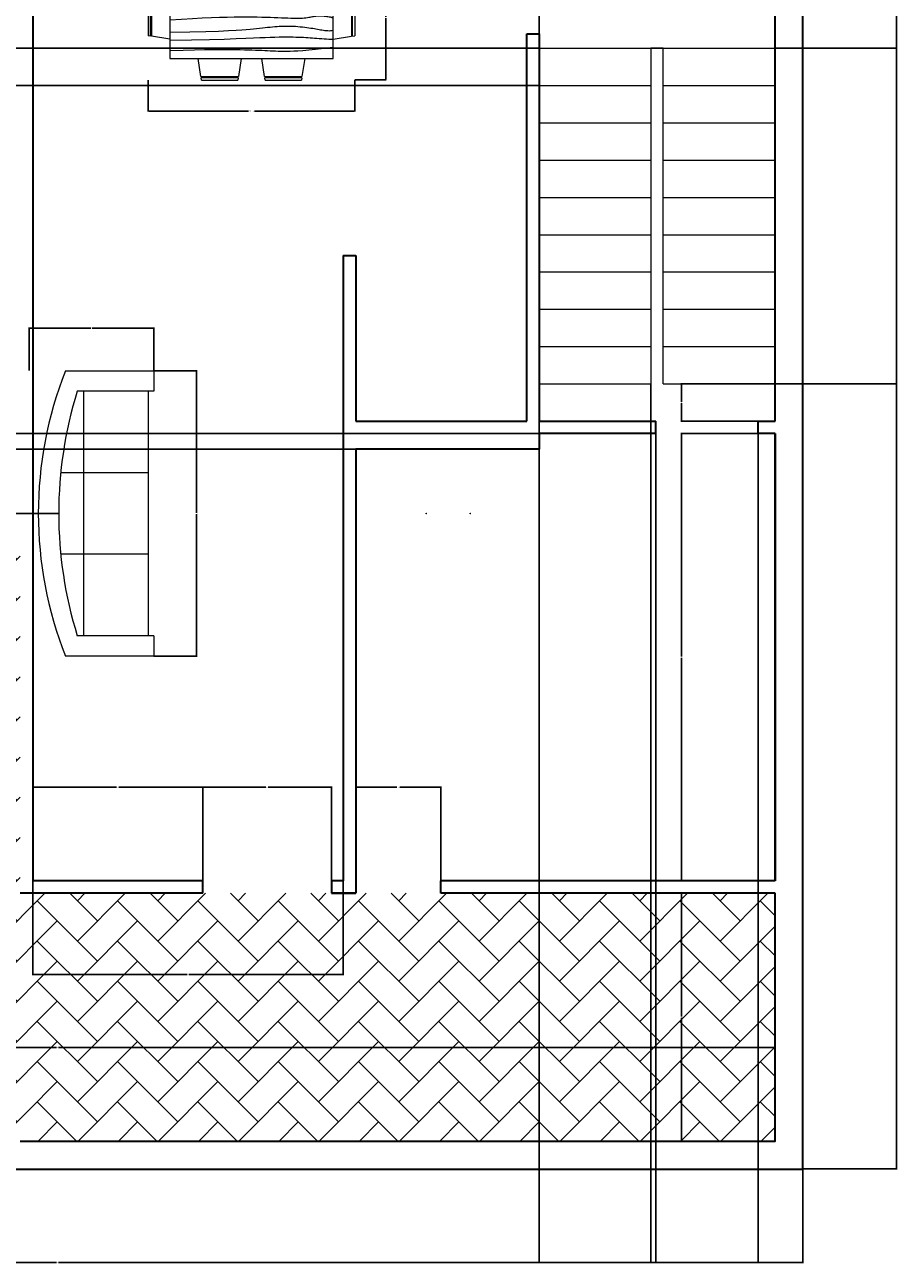
# Model space of a CAD drawing. Units: feet. Extents: x 2335 to 2876, y 491 to 1152.
# Tile 2 of 4: x 2595 to 2876, y 491 to 890. Entities that reach past the tile are written whole.
import ezdxf

# ---------------------------------------------------------------- set-up
doc = ezdxf.new("R2010")
doc.units = ezdxf.units.FT
for name, color, linetype, lineweight in [('A-ANNO-DIMS', 2, 'Continuous', 18), ('A-FLOR-STRS', 4, 'Continuous', 18), ('A-FURN', 8, 'Continuous', 18), ('A-WALL', 7, 'Continuous', 35), ('C-PROP', 3, 'Continuous', 35), ('C-PVMT-PATT', 252, 'Continuous', 13)]:
    doc.layers.add(name, color=color, linetype=linetype, lineweight=lineweight)
doc.styles.get("Standard").update_dxf_attribs({"font": 'arial.ttf'})
doc.dimstyles.get("Standard").update_dxf_attribs({"dimtxt": 0.18, "dimasz": 0.18, "dimexe": 0.18, "dimexo": 0.0625, "dimgap": 0.09, "dimtad": 0, "dimtih": 1, "dimtoh": 1, "dimdec": 4, "dimzin": 0, "dimdsep": 46, "dimlunit": 4, "dimtxsty": 'Standard', "dimcen": 0.09, "dimadec": 0, "dimazin": 0, "dimtfac": 1, "dimtdec": 4, "dimtofl": 0, "dimtmove": 0, "dimatfit": 3, "dimfxl": 1, "dimtolj": 1, "dimtzin": 0, "dimarcsym": 0})

# ---------------------------------------------------------------- blocks, each defined once
blk = doc.blocks.new('Dining Set - 36 x 72 in.')
for p, q in [((-22, 27.5), (-22.1562, 26.50042)), ((-22, 27.5), (-6, 27.5)), ((-5.8437, 26.49966), (-6, 27.5)), ((6, 27.5), (5.8438, 26.50042)), ((6, 27.5), (22, 27.5)), ((22.1563, 26.49966), (22, 27.5)), ((-22.2343, 26.00059), (-23.4847, 17.99762)), ((-22.2304, 26), (-5.7608, 26)), ((-5.8416, 26.5), (-22.1534, 26.5)), ((-4.5152, 17.99762), (-5.7655, 25.99926)), ((5.7657, 26.00059), (4.5153, 17.99762)), ((5.7696, 26), (22.2392, 26)), ((22.1584, 26.5), (5.8466, 26.5)), ((23.4848, 17.99762), (22.2345, 25.99926)), ((36, 18), (-36, 18)), ((-36, 18), (-36, -18)), ((36, -18), (36, 18)), ((-45.5, 8), (-44.5004, 8.15617)), ((-45.5, 8), (-45.5, -8)), ((-44.5, -8.15843), (-44.5, 8.15338)), ((-44.0006, 8.23428), (-35.9976, 9.48474)), ((-44, 8.23041), (-44, -8.23915)), ((44.0006, 8.23428), (35.9976, 9.48474)), ((44, 8.23041), (44, -8.23915)), ((44.5, -8.15843), (44.5, 8.15338)), ((45.5, 8), (44.5005, 8.15617)), ((45.5, 8), (45.5, -8)), ((-44.4997, -8.15631), (-45.5, -8)), ((-35.9976, -9.48476), (-43.9993, -8.2345)), ((35.9976, -9.48476), (43.9993, -8.2345)), ((44.4997, -8.15631), (45.5, -8)), ((-36, -18), (36, -18)), ((-22.2343, -26.0006), (-23.4847, -17.99762)), ((-4.5152, -17.99762), (-5.7655, -25.99928)), ((5.7657, -26.0006), (4.5153, -17.99762)), ((23.4848, -17.99762), (22.2345, -25.99928)), ((-22.2304, -26), (-5.7608, -26)), ((-22, -27.5), (-22.1562, -26.50044)), ((-5.8416, -26.5), (-22.1534, -26.5)), ((-5.8437, -26.49967), (-6, -27.5)), ((5.7696, -26), (22.2392, -26)), ((6, -27.5), (5.8438, -26.50044)), ((22.1584, -26.5), (5.8466, -26.5)), ((22.1563, -26.49967), (22, -27.5)), ((-22, -27.5), (-6, -27.5)), ((6, -27.5), (22, -27.5))]:
    blk.add_line(p, q)
for points in [[(-36, 15), (-31.1772, 14.97754), (-26.8079, 14.91406), (-22.8538, 14.81543), (-19.276, 14.6875), (-16.0362, 14.53613), (-13.0957, 14.36718), (-10.4159, 14.18652), (-7.9583, 14), (-5.6904, 13.81315), (-3.6035, 13.63021), (-1.6954, 13.45508), (0.0365, 13.29166), (1.5945, 13.14388), (2.9811, 13.01562), (4.1988, 12.9108), (5.25, 12.83333), (6.1393, 12.78613), (6.8802, 12.76823), (7.4883, 12.77767), (7.9792, 12.8125), (8.3685, 12.87077), (8.6719, 12.95052), (8.9049, 13.0498), (9.0833, 13.16666), (9.2205, 13.29899), (9.3216, 13.44401), (9.3895, 13.59879), (9.4271, 13.76041), (9.4373, 13.92594), (9.4232, 14.09245), (9.3875, 14.257), (9.3333, 14.41666), (9.2638, 14.56917), (9.1836, 14.71484), (9.0975, 14.85465), (9.0104, 14.98958), (8.9272, 15.1206), (8.8529, 15.2487), (8.7922, 15.37483), (8.75, 15.5), (8.7305, 15.62467), (8.7344, 15.74739), (8.7617, 15.86621), (8.8125, 15.97916), (8.8867, 16.08431), (8.9844, 16.17968), (9.1055, 16.26334), (9.25, 16.33333), (9.4189, 16.38802), (9.6172, 16.42708), (9.8506, 16.45052), (10.125, 16.45833), (10.4463, 16.45052), (10.8203, 16.42708), (11.2529, 16.38802), (11.75, 16.33333), (12.3184, 16.26318), (12.9694, 16.17838), (13.7151, 16.07991), (14.5677, 15.96875), (15.5395, 15.84586), (16.6426, 15.71224), (17.8893, 15.56884), (19.2917, 15.41666), (20.859, 15.25667), (22.5879, 15.08984), (24.4721, 14.91715), (26.5052, 14.73958), (28.6809, 14.5581), (30.9929, 14.3737), (33.4347, 14.18733), (36, 14)], [(-36, 10), (-28.9766, 10.14274), (-23.1725, 10.20442), (-18.4241, 10.19775), (-14.5677, 10.13541), (-11.4399, 10.03011), (-8.877, 9.89453), (-6.7154, 9.74137), (-4.7917, 9.58333), (-2.9698, 9.43082), (-1.2246, 9.28515), (0.4415, 9.14534), (2.026, 9.01041), (3.5266, 8.87939), (4.9408, 8.7513), (6.266, 8.62516), (7.5, 8.5), (8.6411, 8.37549), (9.6914, 8.2539), (10.6538, 8.13818), (11.5312, 8.03125), (12.3267, 7.93603), (13.043, 7.85547), (13.6831, 7.79248), (14.25, 7.75), (14.7471, 7.7303), (15.1797, 7.73307), (15.5537, 7.75732), (15.875, 7.80208), (16.1494, 7.86637), (16.3828, 7.94922), (16.5811, 8.04964), (16.75, 8.16666), (16.8944, 8.29915), (17.0143, 8.44531), (17.1089, 8.60319), (17.1771, 8.77083), (17.218, 8.94629), (17.2305, 9.1276), (17.2137, 9.31282), (17.1667, 9.5), (17.0895, 9.6875), (16.987, 9.875), (16.8649, 10.0625), (16.7292, 10.25), (16.5856, 10.4375), (16.4401, 10.625), (16.2985, 10.8125), (16.1667, 11), (16.05, 11.18733), (15.9518, 11.3737), (15.8752, 11.5581), (15.8229, 11.73958), (15.798, 11.91715), (15.8034, 12.08984), (15.842, 12.25667), (15.9167, 12.41666), (16.0295, 12.56836), (16.1784, 12.70833), (16.3605, 12.83268), (16.5729, 12.9375), (16.8127, 13.01888), (17.0768, 13.07291), (17.3625, 13.0957), (17.6667, 13.08333), (17.9894, 13.03312), (18.3418, 12.94726), (18.7382, 12.82918), (19.1927, 12.68229), (19.7195, 12.51001), (20.3327, 12.31575), (21.0465, 12.10294), (21.875, 11.875), (22.8357, 11.63354), (23.959, 11.37304), (25.2786, 11.08618), (26.8282, 10.76562), (28.6414, 10.40405), (30.752, 9.99414), (33.1936, 9.52856), (36, 9)], [(-36, 5.5), (-30.7157, 5.3348), (-26.069, 5.20963), (-21.9946, 5.11767), (-18.4271, 5.05208), (-15.3009, 5.00602), (-12.5508, 4.97265), (-10.1112, 4.94515), (-7.9167, 4.91666), (-5.909, 4.88167), (-4.0586, 4.83984), (-2.3429, 4.79215), (-0.7396, 4.73958), (0.7739, 4.6831), (2.22, 4.6237), (3.6213, 4.56233), (5, 4.5), (6.373, 4.43782), (7.7344, 4.3776), (9.0723, 4.32129), (10.375, 4.27083), (11.6309, 4.22819), (12.8281, 4.19531), (13.9551, 4.17415), (15, 4.16666), (15.954, 4.17448), (16.819, 4.19791), (17.6001, 4.23698), (18.3021, 4.29166), (18.9299, 4.36198), (19.4883, 4.44791), (19.9823, 4.54948), (20.4167, 4.66666), (20.7969, 4.79899), (21.1302, 4.94401), (21.4245, 5.09879), (21.6875, 5.26041), (21.9271, 5.42594), (22.1511, 5.59245), (22.3672, 5.757), (22.5834, 5.91666), (22.8065, 6.06868), (23.0404, 6.21093), (23.2879, 6.34147), (23.5521, 6.45833), (23.8358, 6.55957), (24.142, 6.64323), (24.4735, 6.70735), (24.8334, 6.75), (25.2235, 6.76969), (25.642, 6.76692), (26.0858, 6.74267), (26.5521, 6.69791), (27.0379, 6.63362), (27.5404, 6.55078), (28.0565, 6.45036), (28.5834, 6.33333), (29.1242, 6.19987), (29.7071, 6.04687), (30.3661, 5.87044), (31.1354, 5.66666), (32.0493, 5.43164), (33.142, 5.16146), (34.4475, 4.85221), (36, 4.5)], [(-36, -1), (-30.7915, -0.6591), (-26.0195, -0.38216), (-21.6519, -0.16284), (-17.6563, 0.00521), (-14.0005, 0.12833), (-10.6523, 0.21289), (-7.5796, 0.26522), (-4.75, 0.29166), (-2.134, 0.29793), (0.2878, 0.28711), (2.5317, 0.26163), (4.6146, 0.22396), (6.5529, 0.17651), (8.3633, 0.12174), (10.0623, 0.06209), (11.6667, 0), (13.1899, -0.06201), (14.6341, -0.1211), (15.9982, -0.17432), (17.2813, -0.21875), (18.4823, -0.25147), (19.6003, -0.26953), (20.6343, -0.27002), (21.5834, -0.25), (22.4481, -0.20768), (23.2357, -0.14584), (23.9549, -0.06836), (24.6146, 0.02083), (25.2235, 0.11784), (25.7904, 0.21875), (26.3241, 0.31966), (26.8334, 0.41666), (27.3265, 0.50618), (27.8099, 0.58593), (28.2894, 0.65397), (28.7709, 0.70833), (29.2601, 0.74707), (29.763, 0.76823), (30.2855, 0.76985), (30.8334, 0.75), (31.4088, 0.70784), (31.9994, 0.64713), (32.589, 0.57275), (33.1615, 0.48958), (33.7008, 0.4025), (34.1908, 0.3164), (34.6153, 0.23616), (34.9584, 0.16666), (35.2099, 0.11165), (35.3848, 0.07031), (35.504, 0.04069), (35.5886, 0.02083), (35.6594, 0.00879), (35.7377, 0.0026), (35.8442, 0.00032), (36, 0)], [(-36, -6.5), (-27.1843, -6.31267), (-20.084, -6.1263), (-14.469, -5.9419), (-10.1094, -5.76042), (-6.7752, -5.58285), (-4.2363, -5.41016), (-2.2629, -5.24333), (-0.625, -5.08334), (0.8708, -4.93099), (2.2715, -4.78646), (3.5872, -4.64974), (4.8281, -4.52084), (6.0046, -4.39974), (7.127, -4.28646), (8.2053, -4.18099), (9.25, -4.08334), (10.2705, -3.99382), (11.2734, -3.91407), (12.2647, -3.84603), (13.25, -3.79167), (14.2354, -3.75293), (15.2266, -3.73177), (16.2295, -3.73015), (17.25, -3.75), (18.2912, -3.79248), (19.3451, -3.85547), (20.4009, -3.93604), (21.4479, -4.03125), (22.4754, -4.13819), (23.4727, -4.25391), (24.4289, -4.37549), (25.3334, -4.5), (26.1785, -4.62492), (26.9694, -4.74935), (27.7145, -4.87281), (28.4219, -4.99479), (29.1, -5.11483), (29.7572, -5.23242), (30.4016, -5.34709), (31.0417, -5.45834), (31.6837, -5.56437), (32.3262, -5.65821), (32.9658, -5.73153), (33.599, -5.77604), (34.2224, -5.78345), (34.8327, -5.74545), (35.4264, -5.65373), (36, -5.5)], [(-36, -10), (-26.4022, -9.81299), (-18.4675, -9.62891), (-11.9839, -9.45069), (-6.7396, -9.28125), (-2.5226, -9.12354), (0.8789, -8.98047), (3.6769, -8.85498), (6.0833, -8.75), (8.2767, -8.66765), (10.3021, -8.60677), (12.1712, -8.56543), (13.8958, -8.54167), (15.4876, -8.53353), (16.9583, -8.53907), (18.3197, -8.55632), (19.5834, -8.58334), (20.7616, -8.61841), (21.8685, -8.66081), (22.9188, -8.71004), (23.9271, -8.76563), (24.9081, -8.82707), (25.8763, -8.89388), (26.8465, -8.96558), (27.8334, -9.04167), (28.8474, -9.12118), (29.8828, -9.20117), (30.93, -9.27824), (31.9792, -9.34896), (33.0205, -9.40991), (34.0443, -9.45768), (35.0407, -9.48885), (36, -9.5)], [(-36, -14.5), (-30.0881, -14.33513), (-25.0332, -14.21224), (-20.7312, -14.12647), (-17.0781, -14.07292), (-13.97, -14.04671), (-11.3027, -14.04297), (-8.9724, -14.05681), (-6.875, -14.08334), (-4.9224, -14.11833), (-3.0905, -14.16016), (-1.3709, -14.20785), (0.2448, -14.26042), (1.7647, -14.3169), (3.1973, -14.3763), (4.5507, -14.43767), (5.8333, -14.5), (7.0554, -14.5621), (8.235, -14.62175), (9.3922, -14.67652), (10.5469, -14.72396), (11.7192, -14.76164), (12.929, -14.78711), (14.1965, -14.79794), (15.5417, -14.79167), (16.9933, -14.76424), (18.6152, -14.70508), (20.4804, -14.60197), (22.6615, -14.44271), (25.2312, -14.21509), (28.2624, -13.9069), (31.8277, -13.50594), (36, -13)]]:
    blk.add_lwpolyline(points)
blk = doc.blocks.new('Sofa - Roundback 7 ft.')
for p, q in [((-12.00002, -32.4421), (-12.00003, -6.5971)), ((11.99997, -32.4421), (11.99998, -6.5971)), ((-36.000027, -34), (-36.000027, -11.4696)), ((-35.999844, -13.3819), (35.9998, -13.3819)), ((35.99998, -34), (35.99998, -11.4696)), ((-36.000027, -32.4421), (35.99998, -32.4421))]:
    blk.add_line(p, q)
for points in [[(-36.000027, -34), (-42.000027, -34), (-42.000027, -8)], [(41.99998, -8), (41.99998, -34), (35.99998, -34)]]:
    blk.add_lwpolyline(points)
for centre, radius, start, end in [((0, -114.25), 114.25, 68.43141, 111.5686), ((-0.00001, -127.1968), 121.1968, 72.72033, 107.2797)]:
    blk.add_arc(centre, radius, start, end)
blk = doc.blocks.new('*D20')
at = {"layer": 'A-ANNO-DIMS', "color": 0, "lineweight": -2, "transparency": 16777216}
for p, q in [((2634.96, 871.96), (2634.96, 861.86)), ((2701.49, 871.96), (2701.49, 861.86)), ((2635.14, 862.04), (2667.26, 862.04)), ((2701.31, 862.04), (2669.2, 862.04))]:
    blk.add_line(p, q, dxfattribs=at)
at = {"layer": 'A-ANNO-DIMS', "color": 0, "transparency": 16777216}
for points in [[(2635.14, 862.07), (2635.14, 862.01), (2634.96, 862.04)], [(2701.31, 862.07), (2701.31, 862.01), (2701.49, 862.04)]]:
    blk.add_solid(points, dxfattribs=at)
at = {"layer": 'Defpoints', "color": 0, "transparency": 16777216}
for p in [(2634.96, 872.02), (2701.49, 872.02), (2701.49, 862.04)]:
    blk.add_point(p, dxfattribs=at)
at = {"layer": 'A-ANNO-DIMS', "color": 0, "transparency": 16777216, "insert": (2668.23, 862.04), "char_height": 0.18, "attachment_point": 5}
blk.add_mtext('\\A1;DINING SET 67', dxfattribs=at)
blk = doc.blocks.new('*D21')
at = {"layer": 'A-ANNO-DIMS', "color": 0, "lineweight": -2, "transparency": 16777216}
for p, q in [((2701.56, 912.23), (2711.65, 912.23)), ((2711.47, 912.05), (2711.47, 892.31)), ((2711.47, 872.2), (2711.47, 891.94)), ((2701.56, 872.02), (2711.65, 872.02))]:
    blk.add_line(p, q, dxfattribs=at)
at = {"layer": 'A-ANNO-DIMS', "color": 0, "transparency": 16777216}
for points in [[(2711.44, 912.05), (2711.5, 912.05), (2711.47, 912.23)], [(2711.44, 872.2), (2711.5, 872.2), (2711.47, 872.02)]]:
    blk.add_solid(points, dxfattribs=at)
at = {"layer": 'Defpoints', "color": 0, "transparency": 16777216}
for p in [(2701.49, 912.23), (2711.47, 912.23), (2701.49, 872.02)]:
    blk.add_point(p, dxfattribs=at)
at = {"layer": 'A-ANNO-DIMS', "color": 0, "transparency": 16777216, "insert": (2711.47, 892.13), "char_height": 0.18, "attachment_point": 5}
blk.add_mtext('\\A1;40', dxfattribs=at)
blk = doc.blocks.new('*D22')
at = {"layer": 'A-ANNO-DIMS', "color": 0, "lineweight": -2, "transparency": 16777216}
for p, q in [((2636.85, 778.42), (2650.74, 778.42)), ((2650.56, 778.24), (2650.56, 732.68)), ((2650.56, 686.75), (2650.56, 732.31)), ((2636.85, 686.57), (2650.74, 686.57))]:
    blk.add_line(p, q, dxfattribs=at)
at = {"layer": 'A-ANNO-DIMS', "color": 0, "transparency": 16777216}
for points in [[(2650.53, 778.24), (2650.59, 778.24), (2650.56, 778.42)], [(2650.53, 686.75), (2650.59, 686.75), (2650.56, 686.57)]]:
    blk.add_solid(points, dxfattribs=at)
at = {"layer": 'Defpoints', "color": 0, "transparency": 16777216}
for p in [(2636.79, 778.42), (2650.56, 778.42), (2636.79, 686.57)]:
    blk.add_point(p, dxfattribs=at)
at = {"layer": 'A-ANNO-DIMS', "color": 0, "transparency": 16777216, "insert": (2650.56, 732.49), "char_height": 0.18, "attachment_point": 5}
blk.add_mtext('\\A1;SOFA 92', dxfattribs=at)
blk = doc.blocks.new('*D23')
at = {"layer": 'A-ANNO-DIMS', "color": 0, "lineweight": -2, "transparency": 16777216}
for p, q in [((2596.69, 778.48), (2596.69, 792.37)), ((2596.87, 792.19), (2616.52, 792.19)), ((2636.61, 792.19), (2616.96, 792.19)), ((2636.79, 778.48), (2636.79, 792.37))]:
    blk.add_line(p, q, dxfattribs=at)
at = {"layer": 'A-ANNO-DIMS', "color": 0, "transparency": 16777216}
for points in [[(2596.87, 792.22), (2596.87, 792.16), (2596.69, 792.19)], [(2636.61, 792.22), (2636.61, 792.16), (2636.79, 792.19)]]:
    blk.add_solid(points, dxfattribs=at)
at = {"layer": 'Defpoints', "color": 0, "transparency": 16777216}
for p in [(2596.69, 792.19), (2596.69, 778.42), (2636.79, 778.42)]:
    blk.add_point(p, dxfattribs=at)
at = {"layer": 'A-ANNO-DIMS', "color": 0, "transparency": 16777216, "insert": (2616.74, 792.19), "char_height": 0.18, "attachment_point": 5}
blk.add_mtext('\\A1;40', dxfattribs=at)
blk = doc.blocks.new('*D24')
at = {"layer": 'A-ANNO-DIMS', "color": 0, "lineweight": -2, "transparency": 16777216}
for p, q in [((2365.8, 521.42), (2365.8, 491.16)), ((2845.8, 521.42), (2845.8, 491.16)), ((2365.98, 491.34), (2605.5, 491.34)), ((2845.62, 491.34), (2606.09, 491.34))]:
    blk.add_line(p, q, dxfattribs=at)
at = {"layer": 'A-ANNO-DIMS', "color": 0, "transparency": 16777216}
for points in [[(2365.98, 491.37), (2365.98, 491.31), (2365.8, 491.34)], [(2845.62, 491.37), (2845.62, 491.31), (2845.8, 491.34)]]:
    blk.add_solid(points, dxfattribs=at)
at = {"layer": 'Defpoints', "color": 0, "transparency": 16777216}
for p in [(2365.8, 521.49), (2845.8, 521.49), (2845.8, 491.34)]:
    blk.add_point(p, dxfattribs=at)
at = {"layer": 'A-ANNO-DIMS', "color": 0, "transparency": 16777216, "insert": (2605.8, 491.34), "char_height": 0.18, "attachment_point": 5}
blk.add_mtext('\\A1;480', dxfattribs=at)
blk = doc.blocks.new('*D25')
at = {"layer": 'A-ANNO-DIMS', "color": 0, "lineweight": -2, "transparency": 16777216}
for p, q in [((2845.86, 1121.49), (2876.13, 1121.49)), ((2875.95, 1121.31), (2875.95, 821.67)), ((2875.95, 521.67), (2875.95, 821.31)), ((2845.86, 521.49), (2876.13, 521.49))]:
    blk.add_line(p, q, dxfattribs=at)
at = {"layer": 'A-ANNO-DIMS', "color": 0, "transparency": 16777216}
for points in [[(2875.92, 1121.31), (2875.98, 1121.31), (2875.95, 1121.49)], [(2875.92, 521.67), (2875.98, 521.67), (2875.95, 521.49)]]:
    blk.add_solid(points, dxfattribs=at)
at = {"layer": 'Defpoints', "color": 0, "transparency": 16777216}
for p in [(2845.8, 1121.49), (2875.95, 1121.49), (2845.8, 521.49)]:
    blk.add_point(p, dxfattribs=at)
at = {"layer": 'A-ANNO-DIMS', "color": 0, "transparency": 16777216, "insert": (2875.95, 821.49), "char_height": 0.18, "attachment_point": 5}
blk.add_mtext('\\A1;600', dxfattribs=at)
blk = doc.blocks.new('*D26')
at = {"layer": 'A-ANNO-DIMS', "color": 0, "lineweight": -2, "transparency": 16777216}
for p, q in [((2374.8, 530.55), (2374.8, 560.82)), ((2374.98, 560.64), (2605.51, 560.64)), ((2836.62, 560.64), (2606.09, 560.64)), ((2836.8, 530.55), (2836.8, 560.82))]:
    blk.add_line(p, q, dxfattribs=at)
at = {"layer": 'A-ANNO-DIMS', "color": 0, "transparency": 16777216}
for points in [[(2374.98, 560.67), (2374.98, 560.61), (2374.8, 560.64)], [(2836.62, 560.67), (2836.62, 560.61), (2836.8, 560.64)]]:
    blk.add_solid(points, dxfattribs=at)
at = {"layer": 'Defpoints', "color": 0, "transparency": 16777216}
for p in [(2836.8, 560.64), (2374.8, 530.49), (2836.8, 530.49)]:
    blk.add_point(p, dxfattribs=at)
at = {"layer": 'A-ANNO-DIMS', "color": 0, "transparency": 16777216, "insert": (2605.8, 560.64), "char_height": 0.18, "attachment_point": 5}
blk.add_mtext('\\A1;462', dxfattribs=at)
blk = doc.blocks.new('*D30')
at = {"layer": 'A-ANNO-DIMS', "color": 0, "lineweight": -2, "transparency": 16777216}
for p, q in [((2836.73, 610.23), (2806.47, 610.23)), ((2806.65, 610.05), (2806.65, 570.54)), ((2806.65, 530.67), (2806.65, 570.17)), ((2836.73, 530.49), (2806.47, 530.49))]:
    blk.add_line(p, q, dxfattribs=at)
at = {"layer": 'A-ANNO-DIMS', "color": 0, "transparency": 16777216}
for points in [[(2806.62, 610.05), (2806.68, 610.05), (2806.65, 610.23)], [(2806.62, 530.67), (2806.68, 530.67), (2806.65, 530.49)]]:
    blk.add_solid(points, dxfattribs=at)
at = {"layer": 'Defpoints', "color": 0, "transparency": 16777216}
for p in [(2806.65, 610.23), (2836.8, 610.23), (2836.8, 530.49)]:
    blk.add_point(p, dxfattribs=at)
at = {"layer": 'A-ANNO-DIMS', "color": 0, "transparency": 16777216, "insert": (2806.65, 570.36), "char_height": 0.18, "attachment_point": 5}
blk.add_mtext('\\A1;79.74', dxfattribs=at)
blk = doc.blocks.new('*D31')
at = {"layer": 'A-ANNO-DIMS', "color": 0, "lineweight": -2, "transparency": 16777216}
for p, q in [((2597.8, 614.16), (2597.8, 583.9)), ((2697.8, 614.16), (2697.8, 583.9)), ((2597.98, 584.08), (2647.52, 584.08)), ((2697.62, 584.08), (2648.08, 584.08))]:
    blk.add_line(p, q, dxfattribs=at)
at = {"layer": 'A-ANNO-DIMS', "color": 0, "transparency": 16777216}
for points in [[(2597.98, 584.11), (2597.98, 584.05), (2597.8, 584.08)], [(2697.62, 584.11), (2697.62, 584.05), (2697.8, 584.08)]]:
    blk.add_solid(points, dxfattribs=at)
at = {"layer": 'Defpoints', "color": 0, "transparency": 16777216}
for p in [(2597.8, 614.23), (2697.8, 614.23), (2597.8, 584.08)]:
    blk.add_point(p, dxfattribs=at)
at = {"layer": 'A-ANNO-DIMS', "color": 0, "transparency": 16777216, "insert": (2647.8, 584.08), "char_height": 0.18, "attachment_point": 5}
blk.add_mtext('\\A1;100', dxfattribs=at)
blk = doc.blocks.new('*D32')
at = {"layer": 'A-ANNO-DIMS', "color": 0, "lineweight": -2, "transparency": 16777216}
for p, q in [((2597.8, 614.29), (2597.8, 644.56)), ((2597.98, 644.38), (2624.79, 644.38)), ((2652.4, 644.38), (2625.58, 644.38)), ((2652.58, 614.29), (2652.58, 644.56))]:
    blk.add_line(p, q, dxfattribs=at)
at = {"layer": 'A-ANNO-DIMS', "color": 0, "transparency": 16777216}
for points in [[(2597.98, 644.41), (2597.98, 644.35), (2597.8, 644.38)], [(2652.4, 644.41), (2652.4, 644.35), (2652.58, 644.38)]]:
    blk.add_solid(points, dxfattribs=at)
at = {"layer": 'Defpoints', "color": 0, "transparency": 16777216}
for p in [(2652.58, 644.38), (2597.8, 614.23), (2652.58, 614.23)]:
    blk.add_point(p, dxfattribs=at)
at = {"layer": 'A-ANNO-DIMS', "color": 0, "transparency": 16777216, "insert": (2625.19, 644.38), "char_height": 0.18, "attachment_point": 5}
blk.add_mtext('\\A1;54.78', dxfattribs=at)
blk = doc.blocks.new('*D33')
at = {"layer": 'A-ANNO-DIMS', "color": 0, "lineweight": -2, "transparency": 16777216}
for p, q in [((2652.58, 614.29), (2652.58, 644.56)), ((2652.76, 644.38), (2672.9, 644.38)), ((2693.81, 644.38), (2673.66, 644.38)), ((2693.99, 614.29), (2693.99, 644.56))]:
    blk.add_line(p, q, dxfattribs=at)
at = {"layer": 'A-ANNO-DIMS', "color": 0, "transparency": 16777216}
for points in [[(2652.76, 644.41), (2652.76, 644.35), (2652.58, 644.38)], [(2693.81, 644.41), (2693.81, 644.35), (2693.99, 644.38)]]:
    blk.add_solid(points, dxfattribs=at)
at = {"layer": 'Defpoints', "color": 0, "transparency": 16777216}
for p in [(2693.99, 644.38), (2652.58, 614.23), (2693.99, 614.23)]:
    blk.add_point(p, dxfattribs=at)
at = {"layer": 'A-ANNO-DIMS', "color": 0, "transparency": 16777216, "insert": (2673.28, 644.38), "char_height": 0.18, "attachment_point": 5}
blk.add_mtext('\\A1;41.41', dxfattribs=at)
blk = doc.blocks.new('*D34')
at = {"layer": 'A-ANNO-DIMS', "color": 0, "lineweight": -2, "transparency": 16777216}
for p, q in [((2701.8, 614.29), (2701.8, 644.56)), ((2701.98, 644.38), (2715.03, 644.38)), ((2729, 644.38), (2715.96, 644.38)), ((2729.18, 614.29), (2729.18, 644.56))]:
    blk.add_line(p, q, dxfattribs=at)
at = {"layer": 'A-ANNO-DIMS', "color": 0, "transparency": 16777216}
for points in [[(2701.98, 644.41), (2701.98, 644.35), (2701.8, 644.38)], [(2729, 644.41), (2729, 644.35), (2729.18, 644.38)]]:
    blk.add_solid(points, dxfattribs=at)
at = {"layer": 'Defpoints', "color": 0, "transparency": 16777216}
for p in [(2729.18, 644.38), (2701.8, 614.23), (2729.18, 614.23)]:
    blk.add_point(p, dxfattribs=at)
at = {"layer": 'A-ANNO-DIMS', "color": 0, "transparency": 16777216, "insert": (2715.49, 644.38), "char_height": 0.18, "attachment_point": 5}
blk.add_mtext('\\A1;27.386', dxfattribs=at)
blk = doc.blocks.new('*D35')
at = {"layer": 'A-ANNO-DIMS', "color": 0, "lineweight": -2, "transparency": 16777216}
for p, q in [((2836.73, 758.23), (2806.47, 758.23)), ((2806.65, 758.05), (2806.65, 686.41)), ((2806.65, 614.41), (2806.65, 686.05)), ((2836.73, 614.23), (2806.47, 614.23))]:
    blk.add_line(p, q, dxfattribs=at)
at = {"layer": 'A-ANNO-DIMS', "color": 0, "transparency": 16777216}
for points in [[(2806.62, 758.05), (2806.68, 758.05), (2806.65, 758.23)], [(2806.62, 614.41), (2806.68, 614.41), (2806.65, 614.23)]]:
    blk.add_solid(points, dxfattribs=at)
at = {"layer": 'Defpoints', "color": 0, "transparency": 16777216}
for p in [(2806.65, 758.23), (2836.8, 758.23), (2836.8, 614.23)]:
    blk.add_point(p, dxfattribs=at)
at = {"layer": 'A-ANNO-DIMS', "color": 0, "transparency": 16777216, "insert": (2806.65, 686.23), "char_height": 0.18, "attachment_point": 5}
blk.add_mtext('\\A1;144', dxfattribs=at)
blk = doc.blocks.new('*D37')
at = {"layer": 'A-ANNO-DIMS', "color": 0, "lineweight": -2, "transparency": 16777216}
for p, q in [((2760.88, 882.29), (2760.88, 1151.82)), ((2761.06, 1151.64), (2798.45, 1151.64)), ((2836.62, 1151.64), (2799.23, 1151.64)), ((2836.8, 882.29), (2836.8, 1151.82))]:
    blk.add_line(p, q, dxfattribs=at)
at = {"layer": 'A-ANNO-DIMS', "color": 0, "transparency": 16777216}
for points in [[(2761.06, 1151.67), (2761.06, 1151.61), (2760.88, 1151.64)], [(2836.62, 1151.67), (2836.62, 1151.61), (2836.8, 1151.64)]]:
    blk.add_solid(points, dxfattribs=at)
at = {"layer": 'Defpoints', "color": 0, "transparency": 16777216}
for p in [(2836.8, 1151.64), (2760.88, 882.23), (2836.8, 882.23)]:
    blk.add_point(p, dxfattribs=at)
at = {"layer": 'A-ANNO-DIMS', "color": 0, "transparency": 16777216, "insert": (2798.84, 1151.64), "char_height": 0.18, "attachment_point": 5}
blk.add_mtext('\\A1;75.92', dxfattribs=at)
blk = doc.blocks.new('*D38')
at = {"layer": 'A-ANNO-DIMS', "color": 0, "lineweight": -2, "transparency": 16777216}
for p, q in [((2836.86, 882.23), (2876.13, 882.23)), ((2875.95, 882.05), (2875.95, 828.41)), ((2875.95, 774.41), (2875.95, 828.04)), ((2836.86, 774.23), (2876.13, 774.23))]:
    blk.add_line(p, q, dxfattribs=at)
at = {"layer": 'A-ANNO-DIMS', "color": 0, "transparency": 16777216}
for points in [[(2875.92, 882.05), (2875.98, 882.05), (2875.95, 882.23)], [(2875.92, 774.41), (2875.98, 774.41), (2875.95, 774.23)]]:
    blk.add_solid(points, dxfattribs=at)
at = {"layer": 'Defpoints', "color": 0, "transparency": 16777216}
for p in [(2836.8, 882.23), (2875.95, 882.23), (2836.8, 774.23)]:
    blk.add_point(p, dxfattribs=at)
at = {"layer": 'A-ANNO-DIMS', "color": 0, "transparency": 16777216, "insert": (2875.95, 828.23), "char_height": 0.18, "attachment_point": 5}
blk.add_mtext('\\A1;108', dxfattribs=at)
blk = doc.blocks.new('*D39')
at = {"layer": 'A-ANNO-DIMS', "color": 0, "lineweight": -2, "transparency": 16777216}
for p, q in [((2760.82, 882.23), (2335.47, 882.23)), ((2335.65, 882.05), (2335.65, 876.41)), ((2335.65, 870.41), (2335.65, 876.05)), ((2760.82, 870.23), (2335.47, 870.23))]:
    blk.add_line(p, q, dxfattribs=at)
at = {"layer": 'A-ANNO-DIMS', "color": 0, "transparency": 16777216}
for points in [[(2335.62, 882.05), (2335.68, 882.05), (2335.65, 882.23)], [(2335.62, 870.41), (2335.68, 870.41), (2335.65, 870.23)]]:
    blk.add_solid(points, dxfattribs=at)
at = {"layer": 'Defpoints', "color": 0, "transparency": 16777216}
for p in [(2335.65, 882.23), (2760.88, 882.23), (2760.88, 870.23)]:
    blk.add_point(p, dxfattribs=at)
at = {"layer": 'A-ANNO-DIMS', "color": 0, "transparency": 16777216, "insert": (2335.65, 876.23), "char_height": 0.18, "attachment_point": 5}
blk.add_mtext('\\A1;12', dxfattribs=at)
blk = doc.blocks.new('*D40')
at = {"layer": 'A-ANNO-DIMS', "color": 0, "lineweight": -2, "transparency": 16777216}
for p, q in [((2760.88, 774.16), (2760.88, 491.16)), ((2796.84, 774.16), (2796.84, 491.16)), ((2761.06, 491.34), (2778.46, 491.34)), ((2796.66, 491.34), (2779.25, 491.34))]:
    blk.add_line(p, q, dxfattribs=at)
at = {"layer": 'A-ANNO-DIMS', "color": 0, "transparency": 16777216}
for points in [[(2761.06, 491.37), (2761.06, 491.31), (2760.88, 491.34)], [(2796.66, 491.37), (2796.66, 491.31), (2796.84, 491.34)]]:
    blk.add_solid(points, dxfattribs=at)
at = {"layer": 'Defpoints', "color": 0, "transparency": 16777216}
for p in [(2760.88, 774.23), (2796.84, 774.23), (2796.84, 491.34)]:
    blk.add_point(p, dxfattribs=at)
at = {"layer": 'A-ANNO-DIMS', "color": 0, "transparency": 16777216, "insert": (2778.86, 491.34), "char_height": 0.18, "attachment_point": 5}
blk.add_mtext('\\A1;35.96', dxfattribs=at)
blk = doc.blocks.new('*D41')
at = {"layer": 'A-ANNO-DIMS', "color": 0, "lineweight": -2, "transparency": 16777216}
for p, q in [((2798.42, 758.16), (2798.42, 491.16)), ((2831.4, 758.16), (2831.4, 491.16)), ((2798.6, 491.34), (2814.51, 491.34)), ((2831.22, 491.34), (2815.3, 491.34))]:
    blk.add_line(p, q, dxfattribs=at)
at = {"layer": 'A-ANNO-DIMS', "color": 0, "transparency": 16777216}
for points in [[(2798.6, 491.37), (2798.6, 491.31), (2798.42, 491.34)], [(2831.22, 491.37), (2831.22, 491.31), (2831.4, 491.34)]]:
    blk.add_solid(points, dxfattribs=at)
at = {"layer": 'Defpoints', "color": 0, "transparency": 16777216}
for p in [(2798.42, 758.23), (2831.4, 758.23), (2831.4, 491.34)]:
    blk.add_point(p, dxfattribs=at)
at = {"layer": 'A-ANNO-DIMS', "color": 0, "transparency": 16777216, "insert": (2814.91, 491.34), "char_height": 0.18, "attachment_point": 5}
blk.add_mtext('\\A1;32.98', dxfattribs=at)
blk = doc.blocks.new('*D42')
at = {"layer": 'A-ANNO-DIMS', "color": 0, "lineweight": -2, "transparency": 16777216}
for p, q in [((2836.73, 774.23), (2806.47, 774.23)), ((2806.65, 774.05), (2806.65, 768.41)), ((2806.65, 762.41), (2806.65, 768.05)), ((2836.73, 762.23), (2806.47, 762.23))]:
    blk.add_line(p, q, dxfattribs=at)
at = {"layer": 'A-ANNO-DIMS', "color": 0, "transparency": 16777216}
for points in [[(2806.62, 774.05), (2806.68, 774.05), (2806.65, 774.23)], [(2806.62, 762.41), (2806.68, 762.41), (2806.65, 762.23)]]:
    blk.add_solid(points, dxfattribs=at)
at = {"layer": 'Defpoints', "color": 0, "transparency": 16777216}
for p in [(2806.65, 774.23), (2836.8, 774.23), (2836.8, 762.23)]:
    blk.add_point(p, dxfattribs=at)
at = {"layer": 'A-ANNO-DIMS', "color": 0, "transparency": 16777216, "insert": (2806.65, 768.23), "char_height": 0.18, "attachment_point": 5}
blk.add_mtext('\\A1;12', dxfattribs=at)
blk = doc.blocks.new('*D43')
at = {"layer": 'A-ANNO-DIMS', "color": 0, "lineweight": -2, "transparency": 16777216}
for p, q in [((2760.82, 758.23), (2335.47, 758.23)), ((2335.65, 758.05), (2335.65, 755.91)), ((2335.65, 753.41), (2335.65, 755.54)), ((2760.82, 753.23), (2335.47, 753.23))]:
    blk.add_line(p, q, dxfattribs=at)
at = {"layer": 'A-ANNO-DIMS', "color": 0, "transparency": 16777216}
for points in [[(2335.62, 758.05), (2335.68, 758.05), (2335.65, 758.23)], [(2335.62, 753.41), (2335.68, 753.41), (2335.65, 753.23)]]:
    blk.add_solid(points, dxfattribs=at)
at = {"layer": 'Defpoints', "color": 0, "transparency": 16777216}
for p in [(2335.65, 758.23), (2760.88, 758.23), (2760.88, 753.23)]:
    blk.add_point(p, dxfattribs=at)
at = {"layer": 'A-ANNO-DIMS', "color": 0, "transparency": 16777216, "insert": (2335.65, 755.73), "char_height": 0.18, "attachment_point": 5}
blk.add_mtext('\\A1;5', dxfattribs=at)
blk = doc.blocks.new('*D70')
at = {"layer": 'A-ANNO-DIMS', "color": 0, "lineweight": -2, "transparency": 16777216}
for p, q in [((2526.66, 732.49), (2605.99, 732.49)), ((2738.6, 732.49), (2738.78, 732.49)), ((2738.69, 732.4), (2738.69, 732.58))]:
    blk.add_line(p, q, dxfattribs=at)
at = {"layer": 'A-ANNO-DIMS', "color": 0, "transparency": 16777216}
blk.add_solid([(2605.99, 732.52), (2605.99, 732.46), (2606.17, 732.49)], dxfattribs=at)
at = {"layer": 'Defpoints', "color": 0, "transparency": 16777216}
for p in [(2606.17, 732.49), (2738.69, 732.49)]:
    blk.add_point(p, dxfattribs=at)
at = {"layer": 'A-ANNO-DIMS', "color": 0, "transparency": 16777216, "insert": (2526.11, 732.49), "char_height": 0.18, "attachment_point": 5}
blk.add_mtext('\\A1;R132.52', dxfattribs=at)
blk = doc.blocks.new('*D71')
at = {"layer": 'A-ANNO-DIMS', "color": 0, "lineweight": -2, "transparency": 16777216}
for p, q in [((2524.65, 732.49), (2599.43, 732.49)), ((2724.44, 732.49), (2724.62, 732.49)), ((2724.53, 732.4), (2724.53, 732.58))]:
    blk.add_line(p, q, dxfattribs=at)
at = {"layer": 'A-ANNO-DIMS', "color": 0, "transparency": 16777216}
blk.add_solid([(2599.43, 732.52), (2599.43, 732.46), (2599.61, 732.49)], dxfattribs=at)
at = {"layer": 'Defpoints', "color": 0, "transparency": 16777216}
for p in [(2599.61, 732.49), (2724.53, 732.49)]:
    blk.add_point(p, dxfattribs=at)
at = {"layer": 'A-ANNO-DIMS', "color": 0, "transparency": 16777216, "insert": (2524.1, 732.49), "char_height": 0.18, "attachment_point": 5}
blk.add_mtext('\\A1;R124.93', dxfattribs=at)

msp = doc.modelspace()

# ---------------------------------------------------------------- hatches: boundary and pattern name
at = {"layer": 'C-PVMT-PATT'}
h = msp.add_hatch(dxfattribs=at)
h.set_pattern_fill('AR-HBONE', color=256, scale=0.09)
h.paths.add_polyline_path([(2593.7974, 722.4872), (2419.7974, 722.4872), (2415.7974, 722.4872), (2374.7967, 722.4872), (2374.7967, 530.4872), (2593.7974, 530.4872), (2597.7974, 530.4872), (2836.7967, 530.4872), (2836.7967, 610.2261), (2729.1837, 610.2261), (2652.5752, 610.2261), (2597.7974, 610.2261), (2593.7974, 610.2261)])

# ---------------------------------------------------------------- linework, layer by layer
at = {"layer": 'A-FLOR-STRS'}
for p, q in [((2760.8783, 882.2261), (2836.7967, 882.2261)), ((2800.8375, 882.2261), (2796.8375, 882.2261)), ((2796.8375, 882.2261), (2796.8375, 774.2261)), ((2800.8375, 774.2261), (2800.8375, 882.2261)), ((2760.8783, 870.2261), (2796.8375, 870.2261)), ((2800.8375, 870.2261), (2836.7967, 870.2261)), ((2760.8783, 858.2261), (2796.8375, 858.2261)), ((2800.8375, 858.2261), (2836.7967, 858.2261)), ((2760.8783, 846.2261), (2796.8375, 846.2261)), ((2800.8375, 846.2261), (2836.7967, 846.2261)), ((2760.8783, 834.2261), (2796.8375, 834.2261)), ((2800.8375, 834.2261), (2836.7967, 834.2261)), ((2760.8783, 822.2261), (2796.8375, 822.2261)), ((2800.8375, 822.2261), (2836.7967, 822.2261)), ((2760.8783, 810.2261), (2796.8375, 810.2261)), ((2800.8375, 810.2261), (2836.7967, 810.2261)), ((2760.8783, 798.2261), (2796.8375, 798.2261)), ((2800.8375, 798.2261), (2836.7967, 798.2261)), ((2760.8783, 786.2261), (2796.8375, 786.2261)), ((2800.8375, 786.2261), (2836.7967, 786.2261)), ((2760.8783, 762.2261), (2760.8783, 774.2261)), ((2760.8783, 774.2261), (2796.8375, 774.2261)), ((2800.8375, 774.2261), (2836.7967, 774.2261))]:
    msp.add_line(p, q, dxfattribs=at)
at = {"layer": 'A-WALL'}
for p, q in [((2597.7974, 918.7975), (2597.7974, 614.2261)), ((2756.8783, 762.2261), (2756.8783, 886.8632)), ((2756.8783, 886.8632), (2760.8783, 886.8632)), ((2760.8783, 886.8632), (2760.8783, 762.2261)), ((2697.7974, 815.4872), (2697.7974, 614.2261)), ((2697.7974, 815.4872), (2701.7974, 815.4872)), ((2701.7974, 815.4872), (2701.7974, 762.2261)), ((2701.7974, 815.4872), (2701.7974, 811.4872)), ((2701.7974, 762.2261), (2756.8783, 762.2261)), ((2760.8783, 762.2261), (2798.4174, 762.2261)), ((2798.4174, 758.2261), (2798.4174, 762.2261)), ((2831.3954, 758.2261), (2831.3954, 762.2261)), ((2831.3954, 762.2261), (2836.7967, 762.2261)), ((2760.8783, 758.2261), (2760.8783, 753.2261)), ((2798.4174, 758.2261), (2760.8783, 758.2261)), ((2836.7967, 758.2261), (2831.3954, 758.2261)), ((2760.8783, 753.2261), (2701.7974, 753.2261)), ((2701.7974, 753.2261), (2701.7974, 614.2261)), ((2652.5752, 614.2261), (2597.7974, 614.2261)), ((2652.5752, 610.2261), (2652.5752, 614.2261)), ((2697.7974, 614.2261), (2693.9852, 614.2261)), ((2693.9852, 614.2261), (2693.9852, 610.2261)), ((2701.7974, 614.2261), (2701.7974, 610.2261)), ((2836.7967, 614.2261), (2729.1837, 614.2261)), ((2729.1837, 610.2261), (2729.1837, 614.2261)), ((2597.7974, 610.2261), (2593.7974, 610.2261)), ((2652.5752, 610.2261), (2597.7974, 610.2261)), ((2701.7974, 610.2261), (2693.9852, 610.2261)), ((2693.9852, 610.2261), (2701.7974, 610.2261)), ((2836.7967, 610.2261), (2729.1837, 610.2261))]:
    msp.add_line(p, q, dxfattribs=at)
at = {"layer": 'C-PROP'}
for p, q in [((2836.7967, 758.2261), (2836.7967, 614.2261)), ((2593.7974, 530.4872), (2597.7974, 530.4872))]:
    msp.add_line(p, q, dxfattribs=at)
msp.add_lwpolyline([(2845.7967, 521.4872), (2845.7967, 1121.4872), (2365.7967, 1121.4872), (2365.7967, 521.4872)], close=True, dxfattribs=at)
for points in [[(2836.7967, 762.2261), (2836.7967, 945.7975)], [(2836.7967, 614.2261), (2836.7967, 758.2261)], [(2597.7974, 530.4872), (2836.7967, 530.4872), (2836.7967, 610.2261)]]:
    msp.add_lwpolyline(points, dxfattribs=at)

# ---------------------------------------------------------------- block references
at = {"layer": 'A-FURN', "xscale": 0.7311477324397611, "yscale": 0.7311477324397611, "zscale": 0.7311477324397611}
msp.add_blockref('Dining Set - 36 x 72 in.', (2668.2264, 892.1257), dxfattribs=at)
at = {"layer": 'A-FURN', "xscale": 1.093446222204467, "yscale": 1.093446222204467, "zscale": 1.093446222204467, "rotation": 89.99999999999999}
msp.add_blockref('Sofa - Roundback 7 ft.', (2599.6087, 732.4927), dxfattribs=at)

# ---------------------------------------------------------------- dimensions: what is measured, and where the dimension line sits
at = {"layer": 'A-ANNO-DIMS'}
for base, p1, p2, override, picture, middle in [((2836.7967, 1151.6372), (2760.8783, 882.2261), (2836.7967, 882.2261), {"dimdec": 2, "dimlfac": 1, "dimrnd": 0, "dimzin": 0, "dimdsep": 46, "dimlunit": 2}, '*D37', (2798.8375, 1151.6372)), ((2796.8375, 491.3372), (2760.8783, 774.2261), (2796.8375, 774.2261), {"dimdec": 2, "dimlfac": 1, "dimrnd": 0, "dimzin": 0, "dimdsep": 46, "dimlunit": 2}, '*D40', (2778.8579, 491.3372)), ((2831.3954, 491.3372), (2798.4174, 758.2261), (2831.3954, 758.2261), {"dimdec": 2, "dimlfac": 1, "dimrnd": 0, "dimzin": 0, "dimdsep": 46, "dimlunit": 2}, '*D41', (2814.9064, 491.3372)), ((2652.5752, 644.3761), (2597.7974, 614.2261), (2652.5752, 614.2261), {"dimdec": 2, "dimlfac": 1, "dimrnd": 0, "dimzin": 0, "dimdsep": 46, "dimlunit": 2}, '*D32', (2625.1863, 644.3761)), ((2693.9852, 644.3761), (2652.5752, 614.2261), (2693.9852, 614.2261), {"dimdec": 2, "dimlfac": 1, "dimrnd": 0, "dimzin": 0, "dimdsep": 46, "dimlunit": 2}, '*D33', (2673.2802, 644.3761)), ((2729.1837, 644.3761), (2701.7974, 614.2261), (2729.1837, 614.2261), {"dimdec": 3, "dimlfac": 1, "dimrnd": 0, "dimzin": 0, "dimdsep": 46, "dimlunit": 2}, '*D34', (2715.4906, 644.3761)), ((2845.7967, 491.3372), (2365.7967, 521.4872), (2845.7967, 521.4872), {"dimdec": 0, "dimlfac": 1, "dimrnd": 0, "dimzin": 0, "dimdsep": 46, "dimlunit": 2}, '*D24', (2605.7967, 491.3372))]:
    dim = msp.add_linear_dim(base=base, p1=p1, p2=p2, dimstyle='Standard', override=override, dxfattribs=at)
    dim.commit()
    dim.dimension.update_dxf_attribs({"geometry": picture, "text_midpoint": middle})
for base, p1, p2, angle, override, picture, middle in [((2875.9467, 1121.4872), (2845.7967, 521.4872), (2845.7967, 1121.4872), 90, {"dimdec": 0, "dimlfac": 1, "dimrnd": 0, "dimzin": 0, "dimdsep": 46, "dimlunit": 2}, '*D25', (2875.9467, 821.4872)), ((2711.4738, 912.2323), (2701.4936, 872.0191), (2701.4936, 912.2323), 90, {"dimdec": 0, "dimlfac": 1, "dimrnd": 0, "dimzin": 0, "dimdsep": 46, "dimlunit": 2}, '*D21', (2711.4738, 892.1257)), ((2335.6467, 882.2261), (2760.8783, 870.2261), (2760.8783, 882.2261), 90, {"dimdec": 0, "dimlfac": 1, "dimrnd": 0, "dimzin": 0, "dimdsep": 46, "dimlunit": 2}, '*D39', (2335.6467, 876.2261)), ((2875.9467, 882.2261), (2836.7967, 774.2261), (2836.7967, 882.2261), 90, {"dimdec": 0, "dimlfac": 1, "dimrnd": 0, "dimzin": 0, "dimdsep": 46, "dimlunit": 2}, '*D38', (2875.9467, 828.2261)), ((2596.6928, 792.1948), (2636.7858, 778.4174), (2596.6928, 778.4174), 180, {"dimdec": 0, "dimlfac": 1, "dimrnd": 0, "dimzin": 0, "dimdsep": 46, "dimlunit": 2}, '*D23', (2616.7393, 792.1948)), ((2806.6467, 774.2261), (2836.7967, 762.2261), (2836.7967, 774.2261), 90, {"dimdec": 0, "dimlfac": 1, "dimrnd": 0, "dimzin": 0, "dimdsep": 46, "dimlunit": 2}, '*D42', (2806.6467, 768.2261)), ((2335.6467, 758.2261), (2760.8783, 753.2261), (2760.8783, 758.2261), 90, {"dimdec": 0, "dimlfac": 1, "dimrnd": 0, "dimzin": 0, "dimdsep": 46, "dimlunit": 2}, '*D43', (2335.6467, 755.7261)), ((2806.6467, 758.2261), (2836.7967, 614.2261), (2836.7967, 758.2261), 90, {"dimdec": 0, "dimlfac": 1, "dimrnd": 0, "dimzin": 0, "dimdsep": 46, "dimlunit": 2}, '*D35', (2806.6467, 686.2261)), ((2597.7974, 584.0761), (2697.7974, 614.2261), (2597.7974, 614.2261), 180, {"dimdec": 0, "dimlfac": 1, "dimrnd": 0, "dimzin": 0, "dimdsep": 46, "dimlunit": 2}, '*D31', (2647.7974, 584.0761)), ((2806.6467, 610.2261), (2836.7967, 530.4872), (2836.7967, 610.2261), 90, {"dimdec": 2, "dimlfac": 1, "dimrnd": 0, "dimzin": 0, "dimdsep": 46, "dimlunit": 2}, '*D30', (2806.6467, 570.3566)), ((2836.7967, 560.6372), (2374.7967, 530.4872), (2836.7967, 530.4872), 0, {"dimdec": 0, "dimlfac": 1, "dimrnd": 0, "dimzin": 0, "dimdsep": 46, "dimlunit": 2}, '*D26', (2605.7967, 560.6372))]:
    dim = msp.add_linear_dim(base=base, p1=p1, p2=p2, angle=angle, dimstyle='Standard', override=override, dxfattribs=at)
    dim.commit()
    dim.dimension.update_dxf_attribs({"geometry": picture, "text_midpoint": middle})
dim = msp.add_linear_dim(base=(2701.4936, 862.039), p1=(2634.9592, 872.0191), p2=(2701.4936, 872.0191), text='DINING SET <>', dimstyle='Standard', override={"dimdec": 0, "dimlfac": 1, "dimrnd": 0, "dimzin": 0, "dimdsep": 46, "dimlunit": 2}, dxfattribs=at)
dim.commit()
dim.dimension.update_dxf_attribs({"geometry": '*D20', "text_midpoint": (2668.2264, 862.039)})
dim = msp.add_linear_dim(base=(2650.5633, 778.4174), p1=(2636.7858, 686.5679), p2=(2636.7858, 778.4174), angle=90, text='SOFA <>', dimstyle='Standard', override={"dimdec": 0, "dimlfac": 1, "dimrnd": 0, "dimzin": 0, "dimdsep": 46, "dimlunit": 2}, dxfattribs=at)
dim.commit()
dim.dimension.update_dxf_attribs({"geometry": '*D22', "text_midpoint": (2650.5633, 732.4927)})
for center, mpoint, picture, middle in [((2724.5349, 732.4927), (2599.6087, 732.493), '*D71', (2524.6529, 732.4932)), ((2738.6915, 732.4927), (2606.1693, 732.493), '*D70', (2526.656, 732.4932))]:
    dim = msp.add_radius_dim(center=center, mpoint=mpoint, dimstyle='Standard', override={"dimdec": 2, "dimlfac": 1, "dimrnd": 0, "dimzin": 0, "dimdsep": 46, "dimlunit": 2}, dxfattribs=at)
    dim.commit()
    dim.dimension.update_dxf_attribs({"geometry": picture, "text_midpoint": middle, "dimtype": 164})

doc.saveas('drawing.dxf')
